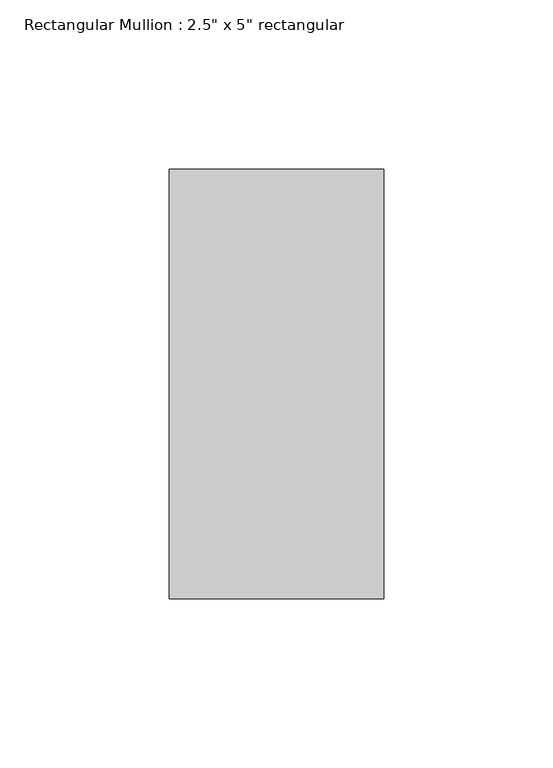
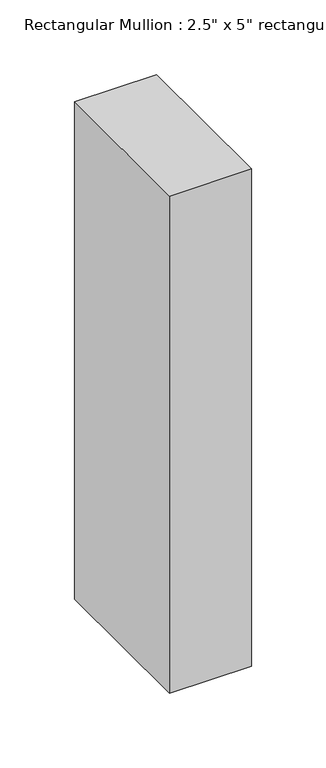
"""IFC4 building model written with IfcOpenShell, lengths in millimetres: member geometry."""

from ifc_helpers import new_model, si_unit, frame, origin, place, context, project, spatial, polyline, outline, extrude, source, transform, mapped, element, save


def member_7cfea1b5(model_context):
    return source(origin(), model_context, "Body", "SweptSolid", [
        extrude(outline(polyline([(0.0, 63.5), (0.0, -63.5), (-63.5, -63.5), (-63.5, 63.5), (0.0, 63.5)])), frame((0.0, 0.0, -406.4), z_axis=(0.0, 0.0, 1.0), x_axis=(1.0, 0.0, 0.0)), (0.0, 0.0, 1.0), 406.4),
    ])


if __name__ == "__main__":
    model = new_model("IFC4")
    model_context = context("Model", 3, world=origin())
    ifc_project = project(units=[si_unit("LENGTHUNIT", "METRE", prefix="MILLI")], contexts=[model_context])
    site = spatial("IfcSite", under=ifc_project)
    building = spatial("IfcBuilding", under=site)
    placement = place(None, origin())
    member_shape = member_7cfea1b5(model_context)
    element("IfcMember", 1, ObjectType="Rectangular Mullion : 2.5\" x 5\" rectangular", at=placement, inside=building, context=model_context, shape_type="MappedRepresentation", body=[
        mapped(member_shape, transform((0.0, 0.0, 0.0), x_axis=(1.0, 0.0, 0.0), y_axis=(0.0, 1.0, 0.0), z_axis=(0.0, 0.0, 1.0))),
    ])
    save(model, "model.ifc")

# Revit data of these elements
# Type "Rectangular Mullion : 2.5\" x 5\" rectangular"
#   built-in parameter 1007304 = 0.416667 (stored number, unit not read)
#   built-in parameter 1007301 = 0.104167 (stored number, unit not read)
#   built-in parameter 1007300 = 0.104167 (stored number, unit not read)
# Element 1 (IfcMember, "Rectangular Mullion : 2.5\" x 5\" rectangular")
#   Materials on its faces: "Aluminum"
# Materials
#   "Aluminum": class "Metal", colour RGB 247 247 247, transparency 0, Description = "Aluminum 6061", Cost = 0
